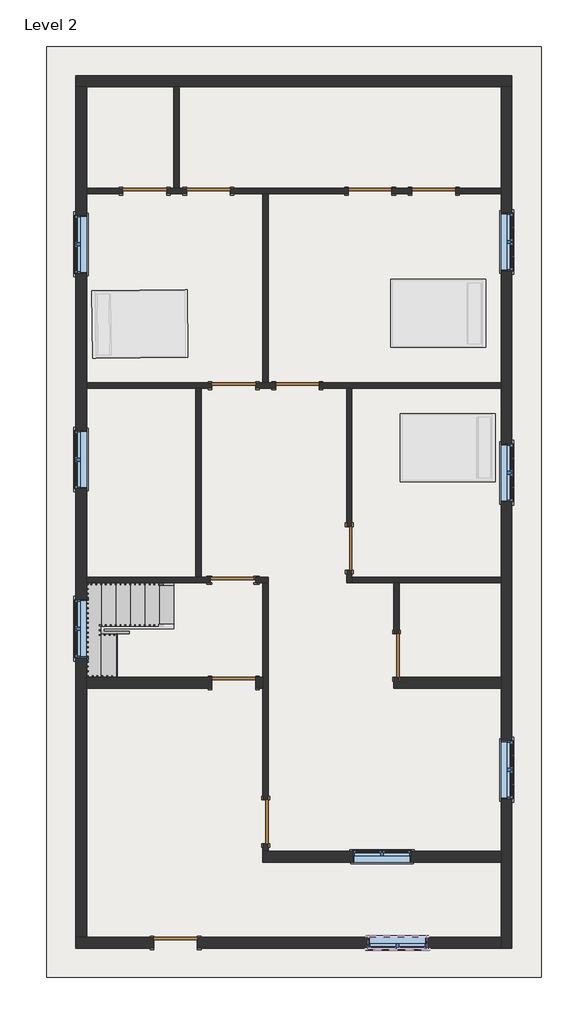
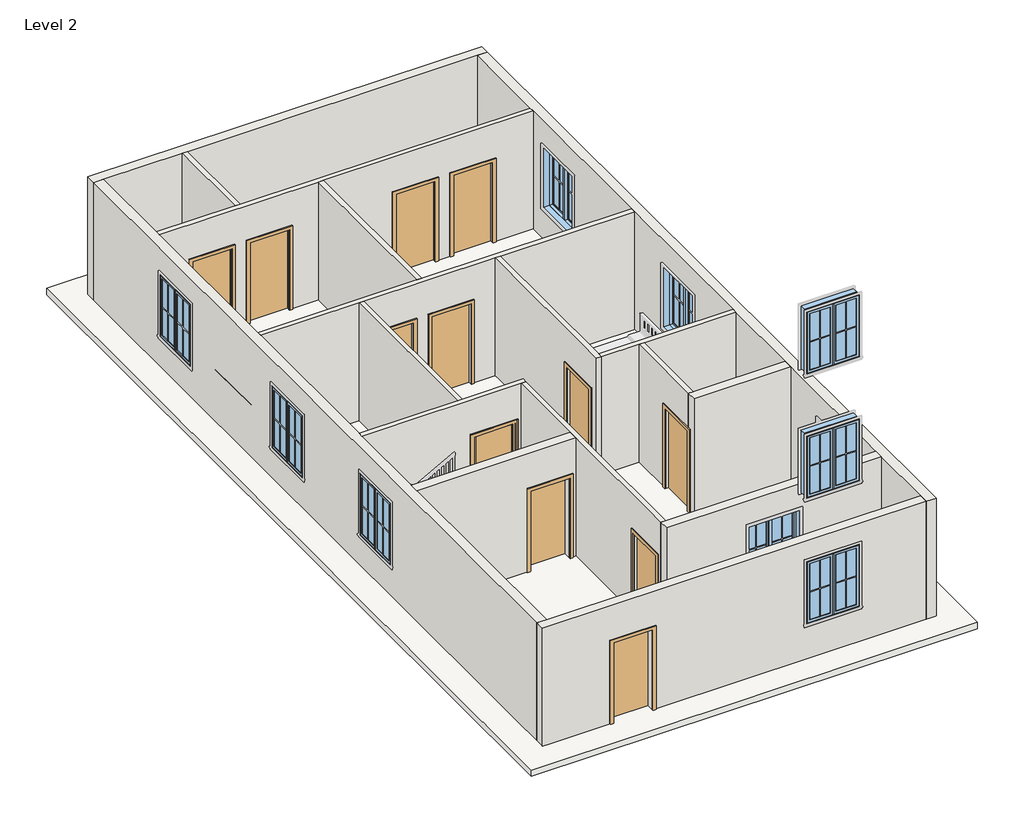
# One storey, part 1 of 2: 17 walls, 13 doors, 10 windows, 1 railing, 1 roof, 1 stair flight.
"""IFC4 building model written with IfcOpenShell, lengths in millimetres."""

from ifc_helpers import new_model, si_unit, frame, origin, place, context, project, spatial, polyline, outline, extrude, faceted_brep, transform, mapped, element, save
from components import door_e5f9f3c4, door_305aa2a5, door_0ca8825f, stair_flight_b60de328, window_8377141f

model = new_model("IFC4")

# Units and contexts
model_context = context("Model", 3, world=origin())
ifc_project = project(units=[si_unit("LENGTHUNIT", "METRE", prefix="MILLI")], contexts=[model_context])

# Site, building, storey
site = spatial("IfcSite", under=ifc_project)
building = spatial("IfcBuilding", under=site)
storey = spatial("IfcBuildingStorey", under=building, Name="Level 2", Elevation=3048.0)

# Doors
placement = place(None, origin())
door_shape = door_e5f9f3c4(model_context)
element("IfcDoor", 1, ObjectType="Single-Flush : 36\" x 84\"", at=placement, inside=storey, context=model_context, shape_type="MappedRepresentation", body=[
    mapped(door_shape, transform((7442.2, 11550.65, 3048.0), x_axis=(1.0, 0.0, 0.0), y_axis=(0.0, 1.0, 0.0), z_axis=(0.0, 0.0, 1.0))),
])
element("IfcDoor", 2, ObjectType="Single-Flush : 36\" x 84\"", at=placement, inside=storey, context=model_context, shape_type="MappedRepresentation", body=[
    mapped(door_shape, transform((2717.8, 11550.65, 3048.0), x_axis=(1.0, 0.0, 0.0), y_axis=(0.0, 1.0, 0.0), z_axis=(0.0, 0.0, 1.0))),
])
element("IfcDoor", 3, ObjectType="Single-Flush : 36\" x 84\"", at=placement, inside=storey, context=model_context, shape_type="MappedRepresentation", body=[
    mapped(door_shape, transform((4584.7, 7473.95, 3048.0), x_axis=(1.0, 0.0, 0.0), y_axis=(0.0, 1.0, 0.0), z_axis=(0.0, 0.0, 1.0))),
])
element("IfcDoor", 4, ObjectType="Single-Flush : 36\" x 84\"", at=placement, inside=storey, context=model_context, shape_type="MappedRepresentation", body=[
    mapped(door_shape, transform((4546.6, 3397.25, 3048.0), x_axis=(1.0, 0.0, 0.0), y_axis=(0.0, 1.0, 0.0), z_axis=(0.0, 0.0, 1.0))),
])
element("IfcDoor", 5, ObjectType="Single-Flush : 36\" x 84\"", at=placement, inside=storey, context=model_context, shape_type="MappedRepresentation", body=[
    mapped(door_shape, transform((4584.7, 3397.25, 3048.0), x_axis=(1.0, 0.0, 0.0), y_axis=(0.0, 1.0, 0.0), z_axis=(0.0, 0.0, 1.0))),
])
element("IfcDoor", 6, ObjectType="Single-Flush : 36\" x 84\"", at=placement, inside=storey, context=model_context, shape_type="MappedRepresentation", body=[
    mapped(door_shape, transform((7004.05, 4064.0, 3048.0), x_axis=(0.0, -1.0, 0.0), y_axis=(1.0, 0.0, 0.0), z_axis=(0.0, 0.0, 1.0))),
])
element("IfcDoor", 7, ObjectType="Single-Flush : 36\" x 84\"", at=placement, inside=storey, context=model_context, shape_type="MappedRepresentation", body=[
    mapped(door_shape, transform((5251.45, -1663.7, 3048.0), x_axis=(0.0, -1.0, 0.0), y_axis=(1.0, 0.0, 0.0), z_axis=(0.0, 0.0, 1.0))),
])
door_2_shape = door_305aa2a5(model_context)
element("IfcDoor", 8, ObjectType="Single-Flush : 36\" x 84\"", at=placement, inside=storey, context=model_context, shape_type="MappedRepresentation", body=[
    mapped(door_2_shape, transform((4051.3, 11550.65, 3048.0), x_axis=(-1.0, 0.0, 0.0), y_axis=(0.0, -1.0, 0.0), z_axis=(0.0, 0.0, 1.0))),
])
element("IfcDoor", 9, ObjectType="Single-Flush : 36\" x 84\"", at=placement, inside=storey, context=model_context, shape_type="MappedRepresentation", body=[
    mapped(door_2_shape, transform((5918.2, 7473.95, 3048.0), x_axis=(-1.0, 0.0, 0.0), y_axis=(0.0, -1.0, 0.0), z_axis=(0.0, 0.0, 1.0))),
])
element("IfcDoor", 10, ObjectType="Single-Flush : 36\" x 84\"", at=placement, inside=storey, context=model_context, shape_type="MappedRepresentation", body=[
    mapped(door_2_shape, transform((7994.65, 1816.1, 3048.0), x_axis=(0.0, 1.0, 0.0), y_axis=(-1.0, 0.0, 0.0), z_axis=(0.0, 0.0, 1.0))),
])
element("IfcDoor", 11, ObjectType="Single-Flush : 36\" x 84\"", at=placement, inside=storey, context=model_context, shape_type="MappedRepresentation", body=[
    mapped(door_2_shape, transform((8775.7, 11550.65, 3048.0), x_axis=(-1.0, 0.0, 0.0), y_axis=(0.0, -1.0, 0.0), z_axis=(0.0, 0.0, 1.0))),
])
door_3_shape = door_0ca8825f(model_context)
element("IfcDoor", 12, ObjectType="Single-Flush : 36\" x 84\"", at=placement, inside=storey, context=model_context, shape_type="MappedRepresentation", body=[
    mapped(door_3_shape, transform((4584.7, 1244.6, 3048.0), x_axis=(1.0, 0.0, 0.0), y_axis=(0.0, 1.0, 0.0), z_axis=(0.0, 0.0, 1.0))),
])
element("IfcDoor", 13, ObjectType="Single-Flush : 36\" x 84\"", at=placement, inside=storey, context=model_context, shape_type="MappedRepresentation", body=[
    mapped(door_3_shape, transform((3365.5, -4203.7, 3048.0), x_axis=(1.0, 0.0, 0.0), y_axis=(0.0, 1.0, 0.0), z_axis=(0.0, 0.0, 1.0))),
])

# Railing
element("IfcRailing", 14, ObjectType="Handrail - Rectangular", at=placement, inside=storey, context=model_context, shape_type="SolidModel", body=[
    faceted_brep([(3327.4, 3289.3, 4131.7333333), (3327.4, 3289.3, 4073.620221), (3327.4, 3340.1, 4073.620221), (3327.4, 3340.1, 4131.7333333), (1803.4, 3289.3, 4978.4), (1790.2363978, 3289.3, 4927.6), (1790.2363978, 3340.1, 4927.6), (1803.4, 3340.1, 4978.4), (1549.4, 3289.3, 4978.4), (1549.4, 3289.3, 4927.6), (1498.6, 3340.1, 4927.6), (1498.6, 3340.1, 4978.4), (1549.4, 1485.9, 4978.4), (1549.4, 1435.1, 4927.6), (1498.6, 1435.1, 4927.6), (1498.6, 1485.9, 4978.4), (1549.4, 1485.9, 5048.9555556), (1549.4, 1435.1, 4998.1555556), (1498.6, 1435.1, 4998.1555556), (1498.6, 1485.9, 5048.9555556), (1549.4, 1409.7, 5048.9555556), (1549.4, 1409.7, 4998.1555556), (1498.6, 1358.9, 4998.1555556), (1498.6, 1358.9, 5048.9555556), (1625.6, 1409.7, 5048.9555556), (1638.7636022, 1409.7, 4998.1555556), (1638.7636022, 1358.9, 4998.1555556), (1625.6, 1358.9, 5048.9555556), (3022.6, 1409.7, 5825.0666667), (3022.6, 1358.9, 5825.0666667), (3022.6, 1358.9, 5766.9535543), (3022.6, 1409.7, 5766.9535543)], [[[0, 1, 2, 3]], [[1, 0, 4, 5]], [[2, 1, 5, 6]], [[3, 2, 6, 7]], [[0, 3, 7, 4]], [[5, 4, 8, 9]], [[6, 5, 9, 10]], [[7, 6, 10, 11]], [[4, 7, 11, 8]], [[9, 8, 12, 13]], [[10, 9, 13, 14]], [[11, 10, 14, 15]], [[8, 11, 15, 12]], [[13, 12, 16, 17]], [[14, 13, 17, 18]], [[15, 14, 18, 19]], [[12, 15, 19, 16]], [[17, 16, 20, 21]], [[18, 17, 21, 22]], [[19, 18, 22, 23]], [[16, 19, 23, 20]], [[21, 20, 24, 25]], [[22, 21, 25, 26]], [[23, 22, 26, 27]], [[20, 23, 27, 24]], [[28, 29, 30, 31]], [[25, 24, 28, 31]], [[26, 25, 31, 30]], [[27, 26, 30, 29]], [[24, 27, 29, 28]]]),
    extrude(outline(polyline([(5729.9118876, 2955.925), (5719.3285543, 2936.875), (4741.3333333, 2936.875), (4741.3333333, 2955.925), (5729.9118876, 2955.925)])), frame((0.0, 1374.775, 0.0), z_axis=(0.0, 1.0, 0.0), x_axis=(0.0, 0.0, 1.0)), (0.0, 0.0, 1.0), 19.05),
    extrude(outline(polyline([(5673.4674432, 2854.325), (5662.8841099, 2835.275), (4741.3333333, 2835.275), (4741.3333333, 2854.325), (5673.4674432, 2854.325)])), frame((0.0, 1374.775, 0.0), z_axis=(0.0, 1.0, 0.0), x_axis=(0.0, 0.0, 1.0)), (0.0, 0.0, 1.0), 19.05),
    extrude(outline(polyline([(5617.0229988, 2752.725), (5606.4396654, 2733.675), (4741.3333333, 2733.675), (4741.3333333, 2752.725), (5617.0229988, 2752.725)])), frame((0.0, 1374.775, 0.0), z_axis=(0.0, 1.0, 0.0), x_axis=(0.0, 0.0, 1.0)), (0.0, 0.0, 1.0), 19.05),
    extrude(outline(polyline([(5560.5785543, 2651.125), (5549.995221, 2632.075), (4572.0, 2632.075), (4572.0, 2651.125), (5560.5785543, 2651.125)])), frame((0.0, 1374.775, 0.0), z_axis=(0.0, 1.0, 0.0), x_axis=(0.0, 0.0, 1.0)), (0.0, 0.0, 1.0), 19.05),
    extrude(outline(polyline([(5504.1341099, 2549.525), (5493.5507765, 2530.475), (4572.0, 2530.475), (4572.0, 2549.525), (5504.1341099, 2549.525)])), frame((0.0, 1374.775, 0.0), z_axis=(0.0, 1.0, 0.0), x_axis=(0.0, 0.0, 1.0)), (0.0, 0.0, 1.0), 19.05),
    extrude(outline(polyline([(5447.6896654, 2447.925), (5437.1063321, 2428.875), (4572.0, 2428.875), (4572.0, 2447.925), (5447.6896654, 2447.925)])), frame((0.0, 1374.775, 0.0), z_axis=(0.0, 1.0, 0.0), x_axis=(0.0, 0.0, 1.0)), (0.0, 0.0, 1.0), 19.05),
    extrude(outline(polyline([(5391.245221, 2346.325), (5380.6618876, 2327.275), (4402.6666667, 2327.275), (4402.6666667, 2346.325), (5391.245221, 2346.325)])), frame((0.0, 1374.775, 0.0), z_axis=(0.0, 1.0, 0.0), x_axis=(0.0, 0.0, 1.0)), (0.0, 0.0, 1.0), 19.05),
    extrude(outline(polyline([(5334.8007765, 2244.725), (5324.2174432, 2225.675), (4402.6666667, 2225.675), (4402.6666667, 2244.725), (5334.8007765, 2244.725)])), frame((0.0, 1374.775, 0.0), z_axis=(0.0, 1.0, 0.0), x_axis=(0.0, 0.0, 1.0)), (0.0, 0.0, 1.0), 19.05),
    extrude(outline(polyline([(5278.3563321, 2143.125), (5267.7729988, 2124.075), (4402.6666667, 2124.075), (4402.6666667, 2143.125), (5278.3563321, 2143.125)])), frame((0.0, 1374.775, 0.0), z_axis=(0.0, 1.0, 0.0), x_axis=(0.0, 0.0, 1.0)), (0.0, 0.0, 1.0), 19.05),
    extrude(outline(polyline([(5221.9118876, 2041.525), (5211.3285543, 2022.475), (4233.3333333, 2022.475), (4233.3333333, 2041.525), (5221.9118876, 2041.525)])), frame((0.0, 1374.775, 0.0), z_axis=(0.0, 1.0, 0.0), x_axis=(0.0, 0.0, 1.0)), (0.0, 0.0, 1.0), 19.05),
    extrude(outline(polyline([(5165.4674432, 1939.925), (5154.8841099, 1920.875), (4233.3333333, 1920.875), (4233.3333333, 1939.925), (5165.4674432, 1939.925)])), frame((0.0, 1374.775, 0.0), z_axis=(0.0, 1.0, 0.0), x_axis=(0.0, 0.0, 1.0)), (0.0, 0.0, 1.0), 19.05),
    extrude(outline(polyline([(5109.0229988, 1838.325), (5098.4396654, 1819.275), (4233.3333333, 1819.275), (4233.3333333, 1838.325), (5109.0229988, 1838.325)])), frame((0.0, 1374.775, 0.0), z_axis=(0.0, 1.0, 0.0), x_axis=(0.0, 0.0, 1.0)), (0.0, 0.0, 1.0), 19.05),
    extrude(outline(polyline([(5052.5785543, 1736.725), (5041.995221, 1717.675), (4064.0, 1717.675), (4064.0, 1736.725), (5052.5785543, 1736.725)])), frame((0.0, 1374.775, 0.0), z_axis=(0.0, 1.0, 0.0), x_axis=(0.0, 0.0, 1.0)), (0.0, 0.0, 1.0), 19.05),
    extrude(outline(polyline([(4996.1341099, 1635.125), (4985.5507765, 1616.075), (4064.0, 1616.075), (4064.0, 1635.125), (4996.1341099, 1635.125)])), frame((0.0, 1374.775, 0.0), z_axis=(0.0, 1.0, 0.0), x_axis=(0.0, 0.0, 1.0)), (0.0, 0.0, 1.0), 19.05),
    extrude(outline(polyline([(1514.475, 1495.425), (1533.525, 1495.425), (1533.525, 1476.375), (1514.475, 1476.375), (1514.475, 1495.425)])), frame((0.0, 0.0, 4064.0), z_axis=(0.0, 0.0, 1.0), x_axis=(1.0, 0.0, 0.0)), (0.0, 0.0, 1.0), 863.6),
    extrude(outline(polyline([(1514.475, 1597.025), (1533.525, 1597.025), (1533.525, 1577.975), (1514.475, 1577.975), (1514.475, 1597.025)])), frame((0.0, 0.0, 4064.0), z_axis=(0.0, 0.0, 1.0), x_axis=(1.0, 0.0, 0.0)), (0.0, 0.0, 1.0), 863.6),
    extrude(outline(polyline([(1514.475, 1698.625), (1533.525, 1698.625), (1533.525, 1679.575), (1514.475, 1679.575), (1514.475, 1698.625)])), frame((0.0, 0.0, 4064.0), z_axis=(0.0, 0.0, 1.0), x_axis=(1.0, 0.0, 0.0)), (0.0, 0.0, 1.0), 863.6),
    extrude(outline(polyline([(1514.475, 1800.225), (1533.525, 1800.225), (1533.525, 1781.175), (1514.475, 1781.175), (1514.475, 1800.225)])), frame((0.0, 0.0, 4064.0), z_axis=(0.0, 0.0, 1.0), x_axis=(1.0, 0.0, 0.0)), (0.0, 0.0, 1.0), 863.6),
    extrude(outline(polyline([(1514.475, 1901.825), (1533.525, 1901.825), (1533.525, 1882.775), (1514.475, 1882.775), (1514.475, 1901.825)])), frame((0.0, 0.0, 4064.0), z_axis=(0.0, 0.0, 1.0), x_axis=(1.0, 0.0, 0.0)), (0.0, 0.0, 1.0), 863.6),
    extrude(outline(polyline([(1514.475, 2003.425), (1533.525, 2003.425), (1533.525, 1984.375), (1514.475, 1984.375), (1514.475, 2003.425)])), frame((0.0, 0.0, 4064.0), z_axis=(0.0, 0.0, 1.0), x_axis=(1.0, 0.0, 0.0)), (0.0, 0.0, 1.0), 863.6),
    extrude(outline(polyline([(1514.475, 2105.025), (1533.525, 2105.025), (1533.525, 2085.975), (1514.475, 2085.975), (1514.475, 2105.025)])), frame((0.0, 0.0, 4064.0), z_axis=(0.0, 0.0, 1.0), x_axis=(1.0, 0.0, 0.0)), (0.0, 0.0, 1.0), 863.6),
    extrude(outline(polyline([(1514.475, 2206.625), (1533.525, 2206.625), (1533.525, 2187.575), (1514.475, 2187.575), (1514.475, 2206.625)])), frame((0.0, 0.0, 4064.0), z_axis=(0.0, 0.0, 1.0), x_axis=(1.0, 0.0, 0.0)), (0.0, 0.0, 1.0), 863.6),
    extrude(outline(polyline([(1514.475, 2308.225), (1533.525, 2308.225), (1533.525, 2289.175), (1514.475, 2289.175), (1514.475, 2308.225)])), frame((0.0, 0.0, 4064.0), z_axis=(0.0, 0.0, 1.0), x_axis=(1.0, 0.0, 0.0)), (0.0, 0.0, 1.0), 863.6),
    extrude(outline(polyline([(1514.475, 2409.825), (1533.525, 2409.825), (1533.525, 2390.775), (1514.475, 2390.775), (1514.475, 2409.825)])), frame((0.0, 0.0, 4064.0), z_axis=(0.0, 0.0, 1.0), x_axis=(1.0, 0.0, 0.0)), (0.0, 0.0, 1.0), 863.6),
    extrude(outline(polyline([(1514.475, 2511.425), (1533.525, 2511.425), (1533.525, 2492.375), (1514.475, 2492.375), (1514.475, 2511.425)])), frame((0.0, 0.0, 4064.0), z_axis=(0.0, 0.0, 1.0), x_axis=(1.0, 0.0, 0.0)), (0.0, 0.0, 1.0), 863.6),
    extrude(outline(polyline([(1514.475, 2613.025), (1533.525, 2613.025), (1533.525, 2593.975), (1514.475, 2593.975), (1514.475, 2613.025)])), frame((0.0, 0.0, 4064.0), z_axis=(0.0, 0.0, 1.0), x_axis=(1.0, 0.0, 0.0)), (0.0, 0.0, 1.0), 863.6),
    extrude(outline(polyline([(1514.475, 2714.625), (1533.525, 2714.625), (1533.525, 2695.575), (1514.475, 2695.575), (1514.475, 2714.625)])), frame((0.0, 0.0, 4064.0), z_axis=(0.0, 0.0, 1.0), x_axis=(1.0, 0.0, 0.0)), (0.0, 0.0, 1.0), 863.6),
    extrude(outline(polyline([(1514.475, 2816.225), (1533.525, 2816.225), (1533.525, 2797.175), (1514.475, 2797.175), (1514.475, 2816.225)])), frame((0.0, 0.0, 4064.0), z_axis=(0.0, 0.0, 1.0), x_axis=(1.0, 0.0, 0.0)), (0.0, 0.0, 1.0), 863.6),
    extrude(outline(polyline([(1514.475, 2917.825), (1533.525, 2917.825), (1533.525, 2898.775), (1514.475, 2898.775), (1514.475, 2917.825)])), frame((0.0, 0.0, 4064.0), z_axis=(0.0, 0.0, 1.0), x_axis=(1.0, 0.0, 0.0)), (0.0, 0.0, 1.0), 863.6),
    extrude(outline(polyline([(1514.475, 3019.425), (1533.525, 3019.425), (1533.525, 3000.375), (1514.475, 3000.375), (1514.475, 3019.425)])), frame((0.0, 0.0, 4064.0), z_axis=(0.0, 0.0, 1.0), x_axis=(1.0, 0.0, 0.0)), (0.0, 0.0, 1.0), 863.6),
    extrude(outline(polyline([(1514.475, 3121.025), (1533.525, 3121.025), (1533.525, 3101.975), (1514.475, 3101.975), (1514.475, 3121.025)])), frame((0.0, 0.0, 4064.0), z_axis=(0.0, 0.0, 1.0), x_axis=(1.0, 0.0, 0.0)), (0.0, 0.0, 1.0), 863.6),
    extrude(outline(polyline([(1514.475, 3222.625), (1533.525, 3222.625), (1533.525, 3203.575), (1514.475, 3203.575), (1514.475, 3222.625)])), frame((0.0, 0.0, 4064.0), z_axis=(0.0, 0.0, 1.0), x_axis=(1.0, 0.0, 0.0)), (0.0, 0.0, 1.0), 863.6),
    extrude(outline(polyline([(1609.725, 3324.225), (1609.725, 3305.175), (1590.675, 3305.175), (1590.675, 3324.225), (1609.725, 3324.225)])), frame((0.0, 0.0, 4064.0), z_axis=(0.0, 0.0, 1.0), x_axis=(1.0, 0.0, 0.0)), (0.0, 0.0, 1.0), 863.6),
    extrude(outline(polyline([(1711.325, 3324.225), (1711.325, 3305.175), (1692.275, 3305.175), (1692.275, 3324.225), (1711.325, 3324.225)])), frame((0.0, 0.0, 4064.0), z_axis=(0.0, 0.0, 1.0), x_axis=(1.0, 0.0, 0.0)), (0.0, 0.0, 1.0), 863.6),
    extrude(outline(polyline([(4914.995221, 1812.925), (4925.5785543, 1793.875), (4064.0, 1793.875), (4064.0, 1812.925), (4914.995221, 1812.925)])), frame((0.0, 3305.175, 0.0), z_axis=(0.0, 1.0, 0.0), x_axis=(0.0, 0.0, 1.0)), (0.0, 0.0, 1.0), 19.05),
    extrude(outline(polyline([(4858.5507765, 1914.525), (4869.1341099, 1895.475), (3894.6666667, 1895.475), (3894.6666667, 1914.525), (4858.5507765, 1914.525)])), frame((0.0, 3305.175, 0.0), z_axis=(0.0, 1.0, 0.0), x_axis=(0.0, 0.0, 1.0)), (0.0, 0.0, 1.0), 19.05),
    extrude(outline(polyline([(4802.1063321, 2016.125), (4812.6896654, 1997.075), (3894.6666667, 1997.075), (3894.6666667, 2016.125), (4802.1063321, 2016.125)])), frame((0.0, 3305.175, 0.0), z_axis=(0.0, 1.0, 0.0), x_axis=(0.0, 0.0, 1.0)), (0.0, 0.0, 1.0), 19.05),
    extrude(outline(polyline([(4745.6618876, 2117.725), (4756.245221, 2098.675), (3894.6666667, 2098.675), (3894.6666667, 2117.725), (4745.6618876, 2117.725)])), frame((0.0, 3305.175, 0.0), z_axis=(0.0, 1.0, 0.0), x_axis=(0.0, 0.0, 1.0)), (0.0, 0.0, 1.0), 19.05),
    extrude(outline(polyline([(4689.2174432, 2219.325), (4699.8007765, 2200.275), (3725.3333333, 2200.275), (3725.3333333, 2219.325), (4689.2174432, 2219.325)])), frame((0.0, 3305.175, 0.0), z_axis=(0.0, 1.0, 0.0), x_axis=(0.0, 0.0, 1.0)), (0.0, 0.0, 1.0), 19.05),
    extrude(outline(polyline([(4632.7729988, 2320.925), (4643.3563321, 2301.875), (3725.3333333, 2301.875), (3725.3333333, 2320.925), (4632.7729988, 2320.925)])), frame((0.0, 3305.175, 0.0), z_axis=(0.0, 1.0, 0.0), x_axis=(0.0, 0.0, 1.0)), (0.0, 0.0, 1.0), 19.05),
    extrude(outline(polyline([(4576.3285543, 2422.525), (4586.9118876, 2403.475), (3725.3333333, 2403.475), (3725.3333333, 2422.525), (4576.3285543, 2422.525)])), frame((0.0, 3305.175, 0.0), z_axis=(0.0, 1.0, 0.0), x_axis=(0.0, 0.0, 1.0)), (0.0, 0.0, 1.0), 19.05),
    extrude(outline(polyline([(4519.8841099, 2524.125), (4530.4674432, 2505.075), (3556.0, 2505.075), (3556.0, 2524.125), (4519.8841099, 2524.125)])), frame((0.0, 3305.175, 0.0), z_axis=(0.0, 1.0, 0.0), x_axis=(0.0, 0.0, 1.0)), (0.0, 0.0, 1.0), 19.05),
    extrude(outline(polyline([(4463.4396654, 2625.725), (4474.0229988, 2606.675), (3556.0, 2606.675), (3556.0, 2625.725), (4463.4396654, 2625.725)])), frame((0.0, 3305.175, 0.0), z_axis=(0.0, 1.0, 0.0), x_axis=(0.0, 0.0, 1.0)), (0.0, 0.0, 1.0), 19.05),
    extrude(outline(polyline([(4406.995221, 2727.325), (4417.5785543, 2708.275), (3556.0, 2708.275), (3556.0, 2727.325), (4406.995221, 2727.325)])), frame((0.0, 3305.175, 0.0), z_axis=(0.0, 1.0, 0.0), x_axis=(0.0, 0.0, 1.0)), (0.0, 0.0, 1.0), 19.05),
    extrude(outline(polyline([(4350.5507765, 2828.925), (4361.1341099, 2809.875), (3386.6666667, 2809.875), (3386.6666667, 2828.925), (4350.5507765, 2828.925)])), frame((0.0, 3305.175, 0.0), z_axis=(0.0, 1.0, 0.0), x_axis=(0.0, 0.0, 1.0)), (0.0, 0.0, 1.0), 19.05),
    extrude(outline(polyline([(4294.1063321, 2930.525), (4304.6896654, 2911.475), (3386.6666667, 2911.475), (3386.6666667, 2930.525), (4294.1063321, 2930.525)])), frame((0.0, 3305.175, 0.0), z_axis=(0.0, 1.0, 0.0), x_axis=(0.0, 0.0, 1.0)), (0.0, 0.0, 1.0), 19.05),
    extrude(outline(polyline([(4237.6618876, 3032.125), (4248.245221, 3013.075), (3386.6666667, 3013.075), (3386.6666667, 3032.125), (4237.6618876, 3032.125)])), frame((0.0, 3305.175, 0.0), z_axis=(0.0, 1.0, 0.0), x_axis=(0.0, 0.0, 1.0)), (0.0, 0.0, 1.0), 19.05),
    extrude(outline(polyline([(4181.2174432, 3133.725), (4191.8007765, 3114.675), (3217.3333333, 3114.675), (3217.3333333, 3133.725), (4181.2174432, 3133.725)])), frame((0.0, 3305.175, 0.0), z_axis=(0.0, 1.0, 0.0), x_axis=(0.0, 0.0, 1.0)), (0.0, 0.0, 1.0), 19.05),
    extrude(outline(polyline([(4124.7729988, 3235.325), (4135.3563321, 3216.275), (3217.3333333, 3216.275), (3217.3333333, 3235.325), (4124.7729988, 3235.325)])), frame((0.0, 3305.175, 0.0), z_axis=(0.0, 1.0, 0.0), x_axis=(0.0, 0.0, 1.0)), (0.0, 0.0, 1.0), 19.05),
    extrude(outline(polyline([(1514.475, 1393.825), (1533.525, 1393.825), (1533.525, 1374.775), (1514.475, 1374.775), (1514.475, 1393.825)])), frame((0.0, 0.0, 4064.0), z_axis=(0.0, 0.0, 1.0), x_axis=(1.0, 0.0, 0.0)), (0.0, 0.0, 1.0), 934.1555556),
    extrude(outline(polyline([(1533.525, 3324.225), (1533.525, 3305.175), (1514.475, 3305.175), (1514.475, 3324.225), (1533.525, 3324.225)])), frame((0.0, 0.0, 4064.0), z_axis=(0.0, 0.0, 1.0), x_axis=(1.0, 0.0, 0.0)), (0.0, 0.0, 1.0), 863.6),
    extrude(outline(polyline([(5766.9535543, 3022.6), (5756.370221, 3003.55), (4741.3333333, 3003.55), (4741.3333333, 3022.6), (5766.9535543, 3022.6)])), frame((0.0, 1374.775, 0.0), z_axis=(0.0, 1.0, 0.0), x_axis=(0.0, 0.0, 1.0)), (0.0, 0.0, 1.0), 19.05),
    extrude(outline(polyline([(4073.620221, 3327.4), (4084.2035543, 3308.35), (3217.3333333, 3308.35), (3217.3333333, 3327.4), (4073.620221, 3327.4)])), frame((0.0, 3305.175, 0.0), z_axis=(0.0, 1.0, 0.0), x_axis=(0.0, 0.0, 1.0)), (0.0, 0.0, 1.0), 19.05),
])

# Roof
element("IfcRoof", 15, ObjectType="Generic - 12\"", at=placement, inside=storey, context=model_context, shape_type="SweptSolid", body=[
    extrude(outline(polyline([(660.4, 14579.6), (11023.6, 14579.6), (11023.6, -4927.6), (660.4, -4927.6), (660.4, 14579.6)])), frame((0.0, 0.0, 3048.0), z_axis=(0.0, 0.0, 1.0), x_axis=(1.0, 0.0, 0.0)), (0.0, 0.0, 1.0), 152.4),
])

# Stair flight
stair_flight_shape = stair_flight_b60de328(model_context)
element("IfcStairFlight", 16, ObjectType="2\" Tread 1\" Nosing 1/4\" Riser", at=placement, inside=storey, context=model_context, shape_type="MappedRepresentation", body=[
    mapped(stair_flight_shape, transform((0.0, 0.0, 0.0), x_axis=(1.0, 0.0, 0.0), y_axis=(0.0, 1.0, 0.0), z_axis=(0.0, 0.0, 1.0))),
])

# Walls
element("IfcWall", 17, ObjectType="Generic - 5\"", at=placement, inside=storey, context=model_context, shape_type="SweptSolid", body=[
    extrude(outline(polyline([(3327.4, 11607.8), (3327.4, 13741.4), (3441.7, 13741.4), (3441.7, 11607.8), (3327.4, 11607.8)])), frame((0.0, 0.0, 3048.0), z_axis=(0.0, 0.0, 1.0), x_axis=(1.0, 0.0, 0.0)), (0.0, 0.0, 1.0), 3048.0),
])
element("IfcWall", 18, ObjectType="Generic - 5\"", at=placement, inside=storey, context=model_context, shape_type="Brep", body=[
    faceted_brep([(7899.4, 11493.5, 3048.0), (8318.5, 11493.5, 3048.0), (8318.5, 11493.5, 5181.6), (9232.9, 11493.5, 5181.6), (9232.9, 11493.5, 3048.0), (10185.4, 11493.5, 3048.0), (10185.4, 11493.5, 6096.0), (5308.6, 11493.5, 6096.0), (5194.3, 11493.5, 6096.0), (1498.6, 11493.5, 6096.0), (1498.6, 11493.5, 3048.0), (2260.6, 11493.5, 3048.0), (2260.6, 11493.5, 5181.6), (3175.0, 11493.5, 5181.6), (3175.0, 11493.5, 3048.0), (3594.1, 11493.5, 3048.0), (3594.1, 11493.5, 5181.6), (4508.5, 11493.5, 5181.6), (4508.5, 11493.5, 3048.0), (5194.3, 11493.5, 3048.0), (5308.6, 11493.5, 3048.0), (6985.0, 11493.5, 3048.0), (6985.0, 11493.5, 5181.6), (7899.4, 11493.5, 5181.6), (8318.5, 11607.8, 5181.6), (8318.5, 11607.8, 3048.0), (7899.4, 11607.8, 3048.0), (7899.4, 11607.8, 5181.6), (6985.0, 11607.8, 5181.6), (6985.0, 11607.8, 3048.0), (4508.5, 11607.8, 3048.0), (4508.5, 11607.8, 5181.6), (3594.1, 11607.8, 5181.6), (3594.1, 11607.8, 3048.0), (3441.7, 11607.8, 3048.0), (3327.4, 11607.8, 3048.0), (3175.0, 11607.8, 3048.0), (3175.0, 11607.8, 5181.6), (2260.6, 11607.8, 5181.6), (2260.6, 11607.8, 3048.0), (1498.6, 11607.8, 3048.0), (1498.6, 11607.8, 6096.0), (3327.4, 11607.8, 6096.0), (3441.7, 11607.8, 6096.0), (10185.4, 11607.8, 6096.0), (10185.4, 11607.8, 3048.0), (9232.9, 11607.8, 3048.0), (9232.9, 11607.8, 5181.6)], [[[0, 1, 2, 3, 4, 5, 6, 7, 8, 9, 10, 11, 12, 13, 14, 15, 16, 17, 18, 19, 20, 21, 22, 23]], [[24, 25, 26, 27, 28, 29, 30, 31, 32, 33, 34, 35, 36, 37, 38, 39, 40, 41, 42, 43, 44, 45, 46, 47]], [[11, 10, 40, 39]], [[30, 29, 21, 20, 19, 18]], [[36, 35, 34, 33, 15, 14]], [[46, 45, 5, 4]], [[26, 25, 1, 0]], [[9, 8, 7, 6, 44, 43, 42, 41]], [[6, 5, 45, 44]], [[10, 9, 41, 40]], [[27, 26, 0, 23]], [[28, 27, 23, 22]], [[29, 28, 22, 21]], [[37, 36, 14, 13]], [[38, 37, 13, 12]], [[39, 38, 12, 11]], [[16, 15, 33, 32]], [[17, 16, 32, 31]], [[18, 17, 31, 30]], [[2, 1, 25, 24]], [[3, 2, 24, 47]], [[4, 3, 47, 46]]]),
])
element("IfcWall", 19, ObjectType="Generic - 5\"", at=placement, inside=storey, context=model_context, shape_type="Brep", body=[
    faceted_brep([(5041.9, 7416.8, 5181.6), (5041.9, 7416.8, 3048.0), (5461.0, 7416.8, 3048.0), (5461.0, 7416.8, 5181.6), (6375.4, 7416.8, 5181.6), (6375.4, 7416.8, 3048.0), (6946.9, 7416.8, 3048.0), (7061.2, 7416.8, 3048.0), (10185.4, 7416.8, 3048.0), (10185.4, 7416.8, 6096.0), (7061.2, 7416.8, 6096.0), (6946.9, 7416.8, 6096.0), (3898.9, 7416.8, 6096.0), (3784.6, 7416.8, 6096.0), (1498.6, 7416.8, 6096.0), (1498.6, 7416.8, 3048.0), (3784.6, 7416.8, 3048.0), (3898.9, 7416.8, 3048.0), (4127.5, 7416.8, 3048.0), (4127.5, 7416.8, 5181.6), (5461.0, 7531.1, 3048.0), (5308.6, 7531.1, 3048.0), (5194.3, 7531.1, 3048.0), (5041.9, 7531.1, 3048.0), (5041.9, 7531.1, 5181.6), (4127.5, 7531.1, 5181.6), (4127.5, 7531.1, 3048.0), (1498.6, 7531.1, 3048.0), (1498.6, 7531.1, 6096.0), (5194.3, 7531.1, 6096.0), (5308.6, 7531.1, 6096.0), (10185.4, 7531.1, 6096.0), (10185.4, 7531.1, 3048.0), (6375.4, 7531.1, 3048.0), (6375.4, 7531.1, 5181.6), (5461.0, 7531.1, 5181.6)], [[[0, 1, 2, 3, 4, 5, 6, 7, 8, 9, 10, 11, 12, 13, 14, 15, 16, 17, 18, 19]], [[20, 21, 22, 23, 24, 25, 26, 27, 28, 29, 30, 31, 32, 33, 34, 35]], [[33, 32, 8, 7, 6, 5]], [[2, 1, 23, 22, 21, 20]], [[18, 17, 16, 15, 27, 26]], [[14, 13, 12, 11, 10, 9, 31, 30, 29, 28]], [[9, 8, 32, 31]], [[15, 14, 28, 27]], [[3, 2, 20, 35]], [[4, 3, 35, 34]], [[5, 4, 34, 33]], [[24, 23, 1, 0]], [[25, 24, 0, 19]], [[26, 25, 19, 18]]]),
])
element("IfcWall", 20, ObjectType="Generic - 5\"", at=placement, inside=storey, context=model_context, shape_type="SweptSolid", body=[
    extrude(outline(polyline([(5194.3, 7531.1), (5194.3, 11493.5), (5308.6, 11493.5), (5308.6, 7531.1), (5194.3, 7531.1)])), frame((0.0, 0.0, 3048.0), z_axis=(0.0, 0.0, 1.0), x_axis=(1.0, 0.0, 0.0)), (0.0, 0.0, 1.0), 3048.0),
])
element("IfcWall", 21, ObjectType="Generic - 5\"", at=placement, inside=storey, context=model_context, shape_type="SweptSolid", body=[
    extrude(outline(polyline([(3784.6, 3454.4), (3784.6, 7416.8), (3898.9, 7416.8), (3898.9, 3454.4), (3784.6, 3454.4)])), frame((0.0, 0.0, 3048.0), z_axis=(0.0, 0.0, 1.0), x_axis=(1.0, 0.0, 0.0)), (0.0, 0.0, 1.0), 3048.0),
])
element("IfcWall", 22, ObjectType="Generic - 5\"", at=placement, inside=storey, context=model_context, shape_type="Brep", body=[
    faceted_brep([(5308.6, 3340.1, 6096.0), (5194.3, 3340.1, 6096.0), (1498.6, 3340.1, 6096.0), (1498.6, 3340.1, 3048.0), (4089.4, 3340.1, 3048.0), (4089.4, 3340.1, 5181.6), (5041.9, 3340.1, 5181.6), (5041.9, 3340.1, 3048.0), (5194.3, 3340.1, 3048.0), (5308.6, 3340.1, 3048.0), (1498.6, 3454.4, 6096.0), (3784.6, 3454.4, 6096.0), (3898.9, 3454.4, 6096.0), (5308.6, 3454.4, 6096.0), (5308.6, 3454.4, 3048.0), (5041.9, 3454.4, 3048.0), (5041.9, 3454.4, 5181.6), (4089.4, 3454.4, 5181.6), (4089.4, 3454.4, 3048.0), (3898.9, 3454.4, 3048.0), (3784.6, 3454.4, 3048.0), (1498.6, 3454.4, 3048.0)], [[[0, 1, 2, 3, 4, 5, 6, 7, 8, 9]], [[10, 11, 12, 13, 14, 15, 16, 17, 18, 19, 20, 21]], [[3, 21, 20, 19, 18, 4]], [[14, 9, 8, 7, 15]], [[2, 1, 0, 13, 12, 11, 10]], [[3, 2, 10, 21]], [[0, 9, 14, 13]], [[5, 17, 16, 6]], [[18, 17, 5, 4]], [[6, 16, 15, 7]]]),
])
element("IfcWall", 23, ObjectType="Generic - 5\"", at=placement, inside=storey, context=model_context, shape_type="Brep", body=[
    faceted_brep([(5194.3, -2120.9, 5181.6), (5194.3, -2120.9, 3048.0), (5194.3, -2286.0, 3048.0), (5194.3, -2286.0, 6096.0), (5194.3, 1130.3, 6096.0), (5194.3, 1358.9, 6096.0), (5194.3, 3340.1, 6096.0), (5194.3, 3340.1, 3048.0), (5194.3, 1358.9, 3048.0), (5194.3, 1130.3, 3048.0), (5194.3, -1206.5, 3048.0), (5194.3, -1206.5, 5181.6), (5308.6, -2286.0, 3048.0), (5308.6, -2120.9, 3048.0), (5308.6, -2120.9, 5181.6), (5308.6, -1206.5, 5181.6), (5308.6, -1206.5, 3048.0), (5308.6, 3340.1, 3048.0), (5308.6, 3340.1, 6096.0), (5308.6, -2286.0, 6096.0)], [[[0, 1, 2, 3, 4, 5, 6, 7, 8, 9, 10, 11]], [[12, 13, 14, 15, 16, 17, 18, 19]], [[2, 1, 13, 12]], [[10, 9, 8, 7, 17, 16]], [[6, 5, 4, 3, 19, 18]], [[7, 6, 18, 17]], [[3, 2, 12, 19]], [[14, 13, 1, 0]], [[15, 14, 0, 11]], [[16, 15, 11, 10]]]),
])
element("IfcWall", 24, ObjectType="Generic - 5\"", at=placement, inside=storey, context=model_context, shape_type="Brep", body=[
    faceted_brep([(6946.9, 3606.8, 5181.6), (6946.9, 3606.8, 3048.0), (6946.9, 3340.1, 3048.0), (6946.9, 3340.1, 6096.0), (6946.9, 7416.8, 6096.0), (6946.9, 7416.8, 3048.0), (6946.9, 4521.2, 3048.0), (6946.9, 4521.2, 5181.6), (7061.2, 3340.1, 3048.0), (7061.2, 3454.4, 3048.0), (7061.2, 3606.8, 3048.0), (7061.2, 3606.8, 5181.6), (7061.2, 4521.2, 5181.6), (7061.2, 4521.2, 3048.0), (7061.2, 7416.8, 3048.0), (7061.2, 7416.8, 6096.0), (7061.2, 3454.4, 6096.0), (7061.2, 3340.1, 6096.0)], [[[0, 1, 2, 3, 4, 5, 6, 7]], [[8, 9, 10, 11, 12, 13, 14, 15, 16, 17]], [[6, 5, 14, 13]], [[2, 1, 10, 9, 8]], [[4, 3, 17, 16, 15]], [[5, 4, 15, 14]], [[3, 2, 8, 17]], [[11, 10, 1, 0]], [[12, 11, 0, 7]], [[13, 12, 7, 6]]]),
])
element("IfcWall", 25, ObjectType="Generic - 5\"", at=placement, inside=storey, context=model_context, shape_type="SweptSolid", body=[
    extrude(outline(polyline([(1358.9, 6096.0), (3340.1, 6096.0), (3340.1, 3048.0), (2273.3, 3048.0), (2273.3, 5181.6), (1358.9, 5181.6), (1358.9, 6096.0)])), frame((7937.5, 0.0, 0.0), z_axis=(1.0, 0.0, 0.0), x_axis=(0.0, 1.0, 0.0)), (0.0, 0.0, 1.0), 114.3),
])
element("IfcWall", 26, ObjectType="Generic - 5\"", at=placement, inside=storey, context=model_context, shape_type="Brep", body=[
    faceted_brep([(7061.2, 3340.1, 3048.0), (7937.5, 3340.1, 3048.0), (8051.8, 3340.1, 3048.0), (10185.4, 3340.1, 3048.0), (10185.4, 3340.1, 6096.0), (8051.8, 3340.1, 6096.0), (7937.5, 3340.1, 6096.0), (7061.2, 3340.1, 6096.0), (7061.2, 3454.4, 3048.0), (7061.2, 3454.4, 6096.0), (10185.4, 3454.4, 6096.0), (10185.4, 3454.4, 3048.0)], [[[0, 1, 2, 3, 4, 5, 6, 7]], [[8, 9, 10, 11]], [[3, 2, 1, 0, 8, 11]], [[7, 6, 5, 4, 10, 9]], [[0, 7, 9, 8]], [[4, 3, 11, 10]]]),
])
element("IfcWall", 27, ObjectType="Generic - 8\"", at=placement, inside=storey, context=model_context, shape_type="Brep", body=[
    faceted_brep([(1270.0, 13741.4, 3048.0), (1498.6, 13741.4, 3048.0), (3327.4, 13741.4, 3048.0), (3441.7, 13741.4, 3048.0), (10185.4, 13741.4, 3048.0), (10414.0, 13741.4, 3048.0), (10414.0, 13741.4, 6096.0), (10185.4, 13741.4, 6096.0), (3441.7, 13741.4, 6096.0), (3327.4, 13741.4, 6096.0), (1498.6, 13741.4, 6096.0), (1270.0, 13741.4, 6096.0), (1270.0, 13970.0, 3048.0), (1270.0, 13970.0, 6096.0), (10414.0, 13970.0, 6096.0), (10414.0, 13970.0, 3048.0)], [[[0, 1, 2, 3, 4, 5, 6, 7, 8, 9, 10, 11]], [[12, 13, 14, 15]], [[5, 4, 3, 2, 1, 0, 12, 15]], [[11, 10, 9, 8, 7, 6, 14, 13]], [[6, 5, 15, 14]], [[0, 11, 13, 12]]]),
])
element("IfcWall", 28, ObjectType="Generic - 8\"", at=placement, inside=storey, context=model_context, shape_type="Brep", body=[
    faceted_brep([(10185.4, 13741.4, 3048.0), (10185.4, 11607.8, 3048.0), (10185.4, 11493.5, 3048.0), (10185.4, 7531.1, 3048.0), (10185.4, 7416.8, 3048.0), (10185.4, 3454.4, 3048.0), (10185.4, 3340.1, 3048.0), (10185.4, 1358.9, 3048.0), (10185.4, 1130.3, 3048.0), (10185.4, -2286.0, 3048.0), (10185.4, -2514.6, 3048.0), (10185.4, -4089.4, 3048.0), (10185.4, -4318.0, 3048.0), (10185.4, -4318.0, 6096.0), (10185.4, -4089.4, 6096.0), (10185.4, -2514.6, 6096.0), (10185.4, -2286.0, 6096.0), (10185.4, 1130.3, 6096.0), (10185.4, 1358.9, 6096.0), (10185.4, 3340.1, 6096.0), (10185.4, 3454.4, 6096.0), (10185.4, 7416.8, 6096.0), (10185.4, 7531.1, 6096.0), (10185.4, 11493.5, 6096.0), (10185.4, 11607.8, 6096.0), (10185.4, 13741.4, 6096.0), (10185.4, 9874.25, 5486.4), (10185.4, 9874.25, 3962.4), (10185.4, 11093.45, 3962.4), (10185.4, 11093.45, 5486.4), (10185.4, 5035.55, 5486.4), (10185.4, 5035.55, 3962.4), (10185.4, 6254.75, 3962.4), (10185.4, 6254.75, 5486.4), (10185.4, -1187.45, 5486.4), (10185.4, -1187.45, 3962.4), (10185.4, 31.75, 3962.4), (10185.4, 31.75, 5486.4), (10414.0, 13741.4, 3048.0), (10414.0, 13741.4, 6096.0), (10414.0, -4318.0, 6096.0), (10414.0, -4318.0, 3048.0), (10414.0, 9874.25, 5486.4), (10414.0, 11093.45, 5486.4), (10414.0, 11093.45, 3962.4), (10414.0, 9874.25, 3962.4), (10414.0, 5035.55, 5486.4), (10414.0, 6254.75, 5486.4), (10414.0, 6254.75, 3962.4), (10414.0, 5035.55, 3962.4), (10414.0, -1187.45, 5486.4), (10414.0, 31.75, 5486.4), (10414.0, 31.75, 3962.4), (10414.0, -1187.45, 3962.4)], [[[0, 1, 2, 3, 4, 5, 6, 7, 8, 9, 10, 11, 12, 13, 14, 15, 16, 17, 18, 19, 20, 21, 22, 23, 24, 25], [26, 27, 28, 29], [30, 31, 32, 33], [34, 35, 36, 37]], [[38, 39, 40, 41], [42, 43, 44, 45], [46, 47, 48, 49], [50, 51, 52, 53]], [[12, 11, 10, 9, 8, 7, 6, 5, 4, 3, 2, 1, 0, 38, 41]], [[25, 24, 23, 22, 21, 20, 19, 18, 17, 16, 15, 14, 13, 40, 39]], [[0, 25, 39, 38]], [[13, 12, 41, 40]], [[27, 26, 42, 45]], [[28, 27, 45, 44]], [[29, 28, 44, 43]], [[26, 29, 43, 42]], [[31, 30, 46, 49]], [[32, 31, 49, 48]], [[33, 32, 48, 47]], [[30, 33, 47, 46]], [[35, 34, 50, 53]], [[36, 35, 53, 52]], [[37, 36, 52, 51]], [[34, 37, 51, 50]]]),
])
element("IfcWall", 29, ObjectType="Generic - 8\"", at=placement, inside=storey, context=model_context, shape_type="Brep", body=[
    faceted_brep([(10185.4, -4089.4, 3048.0), (3822.7, -4089.4, 3048.0), (3822.7, -4089.4, 5181.6), (2908.3, -4089.4, 5181.6), (2908.3, -4089.4, 3048.0), (1498.6, -4089.4, 3048.0), (1270.0, -4089.4, 3048.0), (1270.0, -4089.4, 6096.0), (1498.6, -4089.4, 6096.0), (10185.4, -4089.4, 6096.0), (7404.1, -4089.4, 5594.6550717), (7404.1, -4089.4, 4070.6550717), (8623.3, -4089.4, 4070.6550717), (8623.3, -4089.4, 5594.6550717), (3822.7, -4318.0, 5181.6), (3822.7, -4318.0, 3048.0), (10185.4, -4318.0, 3048.0), (10185.4, -4318.0, 6096.0), (1270.0, -4318.0, 6096.0), (1270.0, -4318.0, 3048.0), (2908.3, -4318.0, 3048.0), (2908.3, -4318.0, 5181.6), (7404.1, -4318.0, 5594.6550717), (8623.3, -4318.0, 5594.6550717), (8623.3, -4318.0, 4070.6550717), (7404.1, -4318.0, 4070.6550717)], [[[0, 1, 2, 3, 4, 5, 6, 7, 8, 9], [10, 11, 12, 13]], [[14, 15, 16, 17, 18, 19, 20, 21], [22, 23, 24, 25]], [[20, 19, 6, 5, 4]], [[16, 15, 1, 0]], [[9, 8, 7, 18, 17]], [[0, 9, 17, 16]], [[7, 6, 19, 18]], [[2, 1, 15, 14]], [[3, 2, 14, 21]], [[4, 3, 21, 20]], [[11, 10, 22, 25]], [[12, 11, 25, 24]], [[13, 12, 24, 23]], [[10, 13, 23, 22]]]),
])
element("IfcWall", 30, ObjectType="Generic - 8\"", at=placement, inside=storey, context=model_context, shape_type="Brep", body=[
    faceted_brep([(1498.6, -4089.4, 3048.0), (1498.6, 1130.3, 3048.0), (1498.6, 1358.9, 3048.0), (1498.6, 3340.1, 3048.0), (1498.6, 3454.4, 3048.0), (1498.6, 7416.8, 3048.0), (1498.6, 7531.1, 3048.0), (1498.6, 11493.5, 3048.0), (1498.6, 11607.8, 3048.0), (1498.6, 13741.4, 3048.0), (1498.6, 13741.4, 6096.0), (1498.6, 11607.8, 6096.0), (1498.6, 11493.5, 6096.0), (1498.6, 7531.1, 6096.0), (1498.6, 7416.8, 6096.0), (1498.6, 3454.4, 6096.0), (1498.6, 3340.1, 6096.0), (1498.6, 1358.9, 6096.0), (1498.6, 1130.3, 6096.0), (1498.6, -4089.4, 6096.0), (1498.6, 6534.15, 5486.4), (1498.6, 6534.15, 3962.4), (1498.6, 5314.95, 3962.4), (1498.6, 5314.95, 5486.4), (1498.6, 11042.65, 5486.4), (1498.6, 11042.65, 3962.4), (1498.6, 9823.45, 3962.4), (1498.6, 9823.45, 5486.4), (1498.6, 2990.85, 5486.4), (1498.6, 2990.85, 3962.4), (1498.6, 1771.65, 3962.4), (1498.6, 1771.65, 5486.4), (1270.0, -4089.4, 3048.0), (1270.0, -4089.4, 6096.0), (1270.0, 13741.4, 6096.0), (1270.0, 13741.4, 3048.0), (1270.0, 6534.15, 5486.4), (1270.0, 5314.95, 5486.4), (1270.0, 5314.95, 3962.4), (1270.0, 6534.15, 3962.4), (1270.0, 11042.65, 5486.4), (1270.0, 9823.45, 5486.4), (1270.0, 9823.45, 3962.4), (1270.0, 11042.65, 3962.4), (1270.0, 2990.85, 5486.4), (1270.0, 1771.65, 5486.4), (1270.0, 1771.65, 3962.4), (1270.0, 2990.85, 3962.4)], [[[0, 1, 2, 3, 4, 5, 6, 7, 8, 9, 10, 11, 12, 13, 14, 15, 16, 17, 18, 19], [20, 21, 22, 23], [24, 25, 26, 27], [28, 29, 30, 31]], [[32, 33, 34, 35], [36, 37, 38, 39], [40, 41, 42, 43], [44, 45, 46, 47]], [[9, 8, 7, 6, 5, 4, 3, 2, 1, 0, 32, 35]], [[19, 18, 17, 16, 15, 14, 13, 12, 11, 10, 34, 33]], [[10, 9, 35, 34]], [[0, 19, 33, 32]], [[21, 20, 36, 39]], [[22, 21, 39, 38]], [[23, 22, 38, 37]], [[20, 23, 37, 36]], [[25, 24, 40, 43]], [[26, 25, 43, 42]], [[27, 26, 42, 41]], [[24, 27, 41, 40]], [[29, 28, 44, 47]], [[30, 29, 47, 46]], [[31, 30, 46, 45]], [[28, 31, 45, 44]]]),
])
element("IfcWall", 31, ObjectType="Generic - 8\"", at=placement, inside=storey, context=model_context, shape_type="SweptSolid", body=[
    extrude(outline(polyline([(5181.6, 5041.9), (3048.0, 5041.9), (3048.0, 5194.3), (6096.0, 5194.3), (6096.0, 1498.6), (3048.0, 1498.6), (3048.0, 4127.5), (5181.6, 4127.5), (5181.6, 5041.9)])), frame((0.0, 1130.3, 0.0), z_axis=(0.0, 1.0, 0.0), x_axis=(0.0, 0.0, 1.0)), (0.0, 0.0, 1.0), 228.6),
])
element("IfcWall", 32, ObjectType="Generic - 8\"", at=placement, inside=storey, context=model_context, shape_type="Brep", body=[
    faceted_brep([(5194.3, -2514.6, 3048.0), (10185.4, -2514.6, 3048.0), (10185.4, -2514.6, 6096.0), (5194.3, -2514.6, 6096.0), (8299.45, -2514.6, 5486.4), (8299.45, -2514.6, 3962.4), (7080.25, -2514.6, 3962.4), (7080.25, -2514.6, 5486.4), (5194.3, -2286.0, 3048.0), (5194.3, -2286.0, 6096.0), (5308.6, -2286.0, 6096.0), (10185.4, -2286.0, 6096.0), (10185.4, -2286.0, 3048.0), (5308.6, -2286.0, 3048.0), (8299.45, -2286.0, 5486.4), (7080.25, -2286.0, 5486.4), (7080.25, -2286.0, 3962.4), (8299.45, -2286.0, 3962.4)], [[[0, 1, 2, 3], [4, 5, 6, 7]], [[8, 9, 10, 11, 12, 13], [14, 15, 16, 17]], [[1, 0, 8, 13, 12]], [[3, 2, 11, 10, 9]], [[0, 3, 9, 8]], [[2, 1, 12, 11]], [[5, 4, 14, 17]], [[6, 5, 17, 16]], [[7, 6, 16, 15]], [[4, 7, 15, 14]]]),
])
element("IfcWall", 33, ObjectType="Generic - 8\"", at=placement, inside=storey, context=model_context, shape_type="Brep", body=[
    faceted_brep([(7937.5, 1130.3, 3048.0), (10185.4, 1130.3, 3048.0), (10185.4, 1130.3, 6096.0), (7937.5, 1130.3, 6096.0), (7937.5, 1358.9, 3048.0), (7937.5, 1358.9, 5181.6), (7937.5, 1358.9, 6096.0), (8051.8, 1358.9, 6096.0), (10185.4, 1358.9, 6096.0), (10185.4, 1358.9, 3048.0)], [[[0, 1, 2, 3]], [[4, 5, 6, 7, 8, 9]], [[1, 0, 4, 9]], [[3, 2, 8, 7, 6]], [[0, 3, 6, 5, 4]], [[2, 1, 9, 8]]]),
])

# Windows
window_shape = window_8377141f(model_context)
element("IfcWindow", 34, ObjectType="Window-Casement-Double : 48\" x 60\"", at=placement, inside=storey, context=model_context, shape_type="MappedRepresentation", body=[
    mapped(window_shape, transform((1384.3, 5924.55, 3048.0), x_axis=(0.0, 1.0, 0.0), y_axis=(-1.0, 0.0, 0.0), z_axis=(0.0, 0.0, 1.0))),
])
element("IfcWindow", 35, ObjectType="Window-Casement-Double : 48\" x 60\"", at=placement, inside=storey, context=model_context, shape_type="MappedRepresentation", body=[
    mapped(window_shape, transform((1384.3, 10433.05, 3048.0), x_axis=(0.0, 1.0, 0.0), y_axis=(-1.0, 0.0, 0.0), z_axis=(0.0, 0.0, 1.0))),
])
element("IfcWindow", 36, ObjectType="Window-Casement-Double : 48\" x 60\"", at=placement, inside=storey, context=model_context, shape_type="MappedRepresentation", body=[
    mapped(window_shape, transform((10299.7, 10483.85, 3048.0), x_axis=(0.0, -1.0, 0.0), y_axis=(1.0, 0.0, 0.0), z_axis=(0.0, 0.0, 1.0))),
])
element("IfcWindow", 37, ObjectType="Window-Casement-Double : 48\" x 60\"", at=placement, inside=storey, context=model_context, shape_type="MappedRepresentation", body=[
    mapped(window_shape, transform((10299.7, 5645.15, 3048.0), x_axis=(0.0, -1.0, 0.0), y_axis=(1.0, 0.0, 0.0), z_axis=(0.0, 0.0, 1.0))),
])
element("IfcWindow", 38, ObjectType="Window-Casement-Double : 48\" x 60\"", at=placement, inside=storey, context=model_context, shape_type="MappedRepresentation", body=[
    mapped(window_shape, transform((10299.7, -577.85, 3048.0), x_axis=(0.0, -1.0, 0.0), y_axis=(1.0, 0.0, 0.0), z_axis=(0.0, 0.0, 1.0))),
])
element("IfcWindow", 39, ObjectType="Window-Casement-Double : 48\" x 60\"", at=placement, inside=storey, context=model_context, shape_type="MappedRepresentation", body=[
    mapped(window_shape, transform((7689.85, -2400.3, 3048.0), x_axis=(1.0, 0.0, 0.0), y_axis=(0.0, 1.0, 0.0), z_axis=(0.0, 0.0, 1.0))),
])
element("IfcWindow", 40, ObjectType="Window-Casement-Double : 48\" x 60\"", at=placement, inside=storey, context=model_context, shape_type="MappedRepresentation", body=[
    mapped(window_shape, transform((1384.3, 2381.25, 3048.0), x_axis=(0.0, 1.0, 0.0), y_axis=(-1.0, 0.0, 0.0), z_axis=(0.0, 0.0, 1.0))),
])
element("IfcWindow", 41, ObjectType="Window-Casement-Double : 48\" x 60\"", at=placement, inside=storey, context=model_context, shape_type="MappedRepresentation", body=[
    mapped(window_shape, transform((8013.7, -4203.7, 3156.2550717), x_axis=(-1.0, 0.0, 0.0), y_axis=(0.0, -1.0, 0.0), z_axis=(0.0, 0.0, 1.0))),
])
element("IfcWindow", 42, ObjectType="Window-Casement-Double : 48\" x 60\"", at=placement, inside=storey, context=model_context, shape_type="MappedRepresentation", body=[
    mapped(window_shape, transform((8013.7, -4203.7, 6241.3309921), x_axis=(-1.0, 0.0, 0.0), y_axis=(0.0, -1.0, 0.0), z_axis=(0.0, 0.0, 1.0))),
])
element("IfcWindow", 43, ObjectType="Window-Casement-Double : 48\" x 60\"", at=placement, inside=storey, context=model_context, shape_type="MappedRepresentation", body=[
    mapped(window_shape, transform((8013.7, -4203.7, 9291.5484942), x_axis=(-1.0, 0.0, 0.0), y_axis=(0.0, -1.0, 0.0), z_axis=(0.0, 0.0, 1.0))),
])

save(model, "model.ifc")

# Revit data of these elements
# Type "Single-Flush : 36\" x 84\""
#   Type Mark = "1"
#   Construction Type Id = "MDOOR"
#   Assembly Code = "C1020"
#   Analytic Construction = "Metal"
#   Thickness = 0' - 2"
#   Heat Transfer Coefficient (U) = 0.651978 BTU/(h·ft²·°F)
#   Height = 7' - 0"
#   Trim Projection Ext = 0' - 1"
#   Trim Projection Int = 0' - 1"
#   Trim Width = 0' - 3"
#   Width = 3' - 0"
#   Define Thermal Properties by = 1
#   Define Thermal Properties by = 1
#   Door Material = Door - Panel
#   Frame Material = Door - Frame
#   Visual Light Transmittance = 0
#   Solar Heat Gain Coefficient = 0
#   Function = (empty or 0)
#   Wall Closure = (empty or 0)
# Type "Handrail - Rectangular"
#   Assembly Code = "C2010400"
#   built-in parameter 1008612 = 0.0416667 (stored number, unit not read)
#   built-in parameter 1008611 = 0.0416667 (stored number, unit not read)
#   built-in parameter 1008609 = 0.333333 (stored number, unit not read)
#   built-in parameter 1008604 = 0.166667 (stored number, unit not read)
#   built-in parameter 1008603 = 0.166667 (stored number, unit not read)
#   Railing Height = 3' - 0"
#   built-in parameter 1008630 = 2
#   built-in parameter 1008610 = 2
#   built-in parameter 1008618 = Baluster - Square : 3/4"
# Type "Generic - 12\""
#   Assembly Code = "B1020"
#   Layers, outside or top first: 0' - 6" no material (function 1)
# Type "Generic - 5\""
#   Assembly Code = "B2010"
#   Layers, outside or top first: 0' - 4 1/2" no material (function 1)
# Type "Generic - 8\""
#   Assembly Code = "B2010"
# Type "Window-Casement-Double : 48\" x 60\""
#   Type Mark = "17"
#   Fire Rating = "0.5h"
#   Assembly Code = "B2020100"
#   Analytic Construction = "Double glazing - domestic"
#   Frame Extension [instance default] = 0' - 0 1/4"
#   Window Inset [instance default] = 0' - 0"
#   Wall Thickness [instance default] = 0' - 6"
#   Interior Wall Closure [instance default] = 0' - 2 1/4"
#   Half Width = 2' - 0"
#   Visual Light Transmittance = 0.81
#   Thermal Resistance (R) = 1.8146 (h·ft²·°F)/BTU
#   Solar Heat Gain Coefficient = 0.76
#   Rough Width = 4' - 0 1/2"
#   Rough Height = 5' - 0 1/2"
#   Height = 5' - 0"
#   Heat Transfer Coefficient (U) = 0.5511 BTU/(h·ft²·°F)
#   Exterior Wall Closure [instance default] = 0' - 1 1/4"
#   Extension Jamb [instance default] = 0' - 2 1/4"
#   Default Sill Height = 3' - 0"
#   Width = 4' - 0"
#   Define Thermal Properties by = 0
#   Muntin Visibility = yes
#   Interior Trim Visibility [instance default] = yes
#   Exterior Trim Visibility [instance default] = yes
#   Extension Jamb Visibility [instance default] = yes
#   Interior Trim Material = Wood - Stained
#   Muntin Pattern = Muntin Pattern_2x2 : Muntin Pattern_2x2
#   Interior Trim = Trim-Window-Interior-Flat : Picture Frame
#   Interior Frame Material = Wood - Stained
#   Glass Panel Material = Glass
#   Exterior Trim Material = Clad - White
#   Exterior Trim = Trim-Window-Exterior-Flat : with Sill
#   Exterior Frame Material = Clad - White
#   Wall Closure = (empty or 0)
# Elements 1, 2, 3, 4, 5, 6, 7, 8, 9, 10, 11, 12, 13 (IfcDoor, "Single-Flush : 36\" x 84\"")
#   Phase Created = New Construction
#   Materials on its faces: "Door - Frame", "Door - Panel"
# Element 14 (IfcRailing, "Handrail - Rectangular")
#   Phase Created = New Construction
# Element 15 (IfcRoof, "Generic - 12\"")
#   built-in parameter 1001705 = 10.5 (stored number, unit not read)
#   built-in parameter 1001710 = 33615
#   Phase Created = New Construction
#   Materials on its faces: "Clad - White", "Default Roof", "Parking Stripe"
# Element 16 (IfcStairFlight, "2\" Tread 1\" Nosing 1/4\" Riser")
#   Phase Created = New Construction
# Elements 17, 18, 19, 20, 21, 22, 23, 24, 25, 26 (IfcWall, "Generic - 5\"")
#   Top Offset = 0' - 0"
#   Base Offset = 0' - 0"
#   wall height = 10' - 0"
#   Phase Created = New Construction
#   Base Constraint = Level 2
#   Top Constraint = Level 3
#   Materials on its faces: "Default Wall"
# Elements 27, 28, 29, 30 (IfcWall, "Generic - 8\"")
#   Top Offset = 0' - 0"
#   Base Offset = 0' - 0"
#   Unconnected Height = 10' - 0"
#   wall height = 10' - 0"
#   Phase Created = New Construction
#   Base Constraint = Level 2
#   Materials on its faces: "Parking Stripe"
# Element 31 (IfcWall, "Generic - 8\"")
#   Top Offset = 0' - 0"
#   Base Offset = 0' - 0"
#   Unconnected Height = 10' - 0"
#   wall height = 10' - 0"
#   Phase Created = New Construction
#   Base Constraint = Level 2
# Elements 32, 33 (IfcWall, "Generic - 8\"")
#   Top Offset = 0' - 0"
#   Base Offset = 0' - 0"
#   Unconnected Height = 10' - 0"
#   wall height = 10' - 0"
#   Phase Created = New Construction
#   Base Constraint = Level 2
#   Materials on its faces: "Default Wall"
# Element 34 (IfcWindow, "Window-Casement-Double : 48\" x 60\"")
#   Mark = "8"
#   Window Inset = 0' - 0"
#   Interior Wall Closure = 0' - 2 1/4"
#   Frame Extension = 0' - 0 1/4"
#   Exterior Wall Closure = 0' - 1 1/4"
#   Interior Trim Visibility = yes
#   Exterior Trim Visibility = yes
#   Phase Created = New Construction
#   Materials on its faces: "Wood - Stained", "Glass", "Clad - White"
# Element 35 (IfcWindow, "Window-Casement-Double : 48\" x 60\"")
#   Mark = "9"
#   Window Inset = 0' - 0"
#   Interior Wall Closure = 0' - 2 1/4"
#   Frame Extension = 0' - 0 1/4"
#   Exterior Wall Closure = 0' - 1 1/4"
#   Interior Trim Visibility = yes
#   Exterior Trim Visibility = yes
#   Phase Created = New Construction
#   Materials on its faces: "Wood - Stained", "Glass", "Clad - White"
# Element 36 (IfcWindow, "Window-Casement-Double : 48\" x 60\"")
#   Mark = "10"
#   Window Inset = 0' - 0"
#   Interior Wall Closure = 0' - 2 1/4"
#   Frame Extension = 0' - 0 1/4"
#   Exterior Wall Closure = 0' - 1 1/4"
#   Interior Trim Visibility = yes
#   Exterior Trim Visibility = yes
#   Phase Created = New Construction
#   Materials on its faces: "Wood - Stained", "Glass", "Clad - White"
# Element 37 (IfcWindow, "Window-Casement-Double : 48\" x 60\"")
#   Mark = "11"
#   Window Inset = 0' - 0"
#   Interior Wall Closure = 0' - 2 1/4"
#   Frame Extension = 0' - 0 1/4"
#   Exterior Wall Closure = 0' - 1 1/4"
#   Interior Trim Visibility = yes
#   Exterior Trim Visibility = yes
#   Phase Created = New Construction
#   Materials on its faces: "Wood - Stained", "Glass", "Clad - White"
# Element 38 (IfcWindow, "Window-Casement-Double : 48\" x 60\"")
#   Mark = "12"
#   Window Inset = 0' - 0"
#   Interior Wall Closure = 0' - 2 1/4"
#   Frame Extension = 0' - 0 1/4"
#   Exterior Wall Closure = 0' - 1 1/4"
#   Interior Trim Visibility = yes
#   Exterior Trim Visibility = yes
#   Phase Created = New Construction
#   Materials on its faces: "Wood - Stained", "Glass", "Clad - White"
# Element 39 (IfcWindow, "Window-Casement-Double : 48\" x 60\"")
#   Mark = "13"
#   Window Inset = 0' - 0"
#   Interior Wall Closure = 0' - 2 1/4"
#   Frame Extension = 0' - 0 1/4"
#   Exterior Wall Closure = 0' - 1 1/4"
#   Interior Trim Visibility = yes
#   Exterior Trim Visibility = yes
#   Phase Created = New Construction
#   Materials on its faces: "Wood - Stained", "Glass", "Clad - White"
# Element 40 (IfcWindow, "Window-Casement-Double : 48\" x 60\"")
#   Mark = "14"
#   Window Inset = 0' - 0"
#   Interior Wall Closure = 0' - 2 1/4"
#   Frame Extension = 0' - 0 1/4"
#   Exterior Wall Closure = 0' - 1 1/4"
#   Interior Trim Visibility = yes
#   Exterior Trim Visibility = yes
#   Phase Created = New Construction
#   Materials on its faces: "Wood - Stained", "Glass", "Clad - White"
# Element 41 (IfcWindow, "Window-Casement-Double : 48\" x 60\"")
#   Mark = "29"
#   Window Inset = 0' - 0"
#   Interior Wall Closure = 0' - 2 1/4"
#   Frame Extension = 0' - 0 1/4"
#   Exterior Wall Closure = 0' - 1 1/4"
#   Interior Trim Visibility = yes
#   Exterior Trim Visibility = yes
#   Phase Created = New Construction
#   Materials on its faces: "Wood - Stained", "Glass", "Clad - White"
# Element 42 (IfcWindow, "Window-Casement-Double : 48\" x 60\"")
#   Mark = "30"
#   Window Inset = 0' - 0"
#   Interior Wall Closure = 0' - 2 1/4"
#   Frame Extension = 0' - 0 1/4"
#   Exterior Wall Closure = 0' - 1 1/4"
#   Interior Trim Visibility = yes
#   Exterior Trim Visibility = yes
#   Phase Created = New Construction
#   Materials on its faces: "Wood - Stained", "Glass", "Clad - White"
# Element 43 (IfcWindow, "Window-Casement-Double : 48\" x 60\"")
#   Mark = "31"
#   Window Inset = 0' - 0"
#   Interior Wall Closure = 0' - 2 1/4"
#   Frame Extension = 0' - 0 1/4"
#   Exterior Wall Closure = 0' - 1 1/4"
#   Interior Trim Visibility = yes
#   Exterior Trim Visibility = yes
#   Phase Created = New Construction
#   Materials on its faces: "Wood - Stained", "Glass", "Clad - White"
# Materials
#   "Door - Panel": class "Wood", colour RGB 210 159 95, transparency 0, Cost = 0
#   "Door - Frame": colour RGB 118 70 51, transparency 0, Cost = 0
#   "Wood - Stained": class "Wood", colour RGB 224 178 126, transparency 0, Cost = 0
#   "Glass": class "Glass", colour RGB 0 128 192, transparency 0.75, Description = "Soda Lime Glass", Cost = 0
#   "Clad - White": class "Wood", colour RGB 242 242 238, transparency 0, Cost = 0
#   "Default Roof": colour RGB 88 101 114, transparency 0, Cost = 0
#   "Parking Stripe": class "Paint", colour RGB 250 250 91, transparency 0, Cost = 0
#   "Default Wall": colour RGB 128 128 128, transparency 0, Cost = 0
